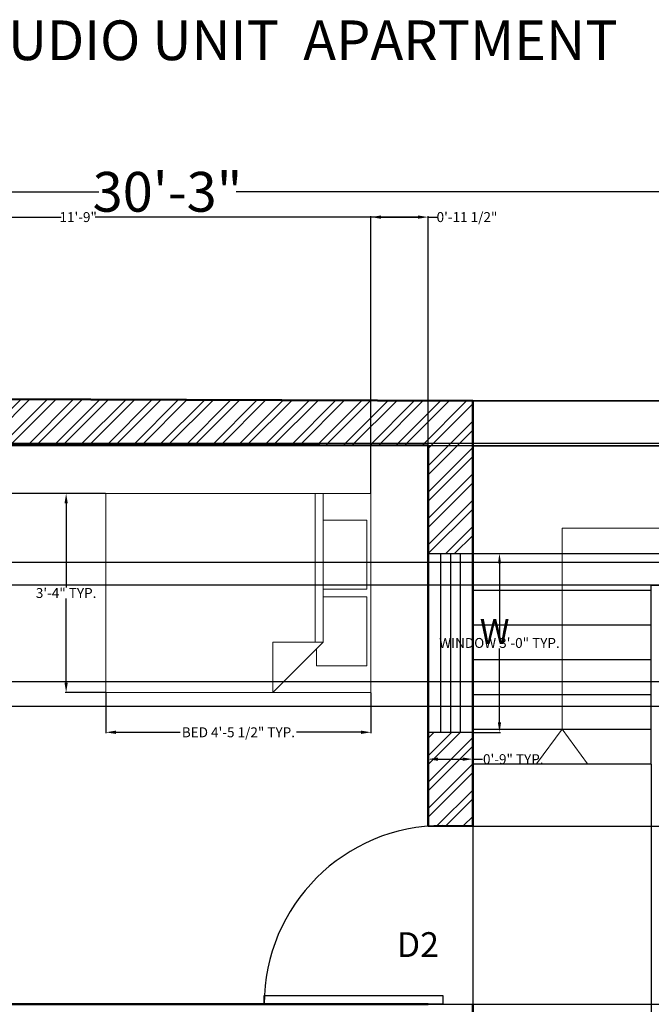
# Model space of a CAD drawing. Units: inches. Extents: x -83 to 408, y 158 to 919.
# Tile 4 of 5: x 111 to 238, y 721 to 919. Entities that reach past the tile are written whole.
import ezdxf

# ---------------------------------------------------------------- set-up
doc = ezdxf.new("R2010")
doc.units = ezdxf.units.IN
doc.header["$MEASUREMENT"] = 0
for name, color, linetype, lineweight in [('A-ANNO-DIMS', 2, 'Continuous', 18), ('A-ANNO-SYMB', 3, 'Continuous', 18), ('A-ANNO-TEXT', 7, 'Continuous', 18), ('A-ANNO-TITL', 7, 'Continuous', 35), ('A-DOOR', 3, 'Continuous', 25), ('A-FLOR-STRS', 7, 'Continuous', 25), ('A-FURN', 8, 'Continuous', 18), ('A-GLAZ', 4, 'Continuous', 25), ('A-WALL', 7, 'Continuous', 50), ('A-WALL-PATT', 252, 'Continuous', 13), ('L-WALL', 7, 'Continuous', 35)]:
    doc.layers.add(name, color=color, linetype=linetype, lineweight=lineweight)
doc.styles.get("Standard").update_dxf_attribs({"font": 'arial.ttf'})
doc.dimstyles.get("Standard").update_dxf_attribs({"dimtxt": 2, "dimasz": 2, "dimexe": 0.18, "dimexo": 0.0625, "dimgap": 0.09, "dimtad": 0, "dimtih": 1, "dimtoh": 1, "dimdec": 0, "dimzin": 0, "dimdsep": 46, "dimlunit": 3, "dimtxsty": 'Standard', "dimcen": 0.09, "dimadec": 0, "dimazin": 0, "dimtfac": 1, "dimtdec": 0, "dimtofl": 0, "dimtmove": 0, "dimatfit": 3, "dimfxl": 1, "dimtolj": 1, "dimtzin": 0, "dimarcsym": 0})

# ---------------------------------------------------------------- blocks, each defined once
blk = doc.blocks.new('Bed - Queen')
for p, q in [((0, -80.00003), (0, 0)), ((0, 0), (59.99999, 0)), ((59.99999, 0), (59.99999, -80.00003)), ((7.99999, -1.2), (28.79998, -1.2)), ((7.99999, -14.4), (7.99999, -1.2)), ((28.79998, -1.2), (28.79998, -14.4)), ((31.19999, -1.2), (51.99999, -1.2)), ((31.19999, -14.4), (31.19999, -1.2)), ((51.99999, -1.2), (51.99999, -16.4)), ((0, -14.4), (44.8, -14.4)), ((59.99999, -29.6), (44.8, -14.4)), ((44.8, -14.4), (44.8, -29.6)), ((44.8, -16.8), (0, -16.8)), ((51.99999, -16.4), (46.79936, -16.4)), ((44.8, -29.6), (59.99999, -29.6)), ((59.99999, -80.00003), (0, -80.00003))]:
    blk.add_line(p, q)
blk = doc.blocks.new('*U13')
for p, q in [((0, 0), (0, -6)), ((36, 0), (36, -6))]:
    blk.add_line(p, q)
blk.add_lwpolyline([(0, 0), (0, 36), (1.75, 36), (1.75, 0)], close=True)
blk.add_arc((0, 0), 36, 0, 90)
blk = doc.blocks.new('*D18')
at = {"layer": 'A-ANNO-DIMS', "color": 0, "lineweight": -2, "transparency": 16777216}
for p, q in [((-40.81, 843.26), (-40.81, 884.97)), ((-38.81, 884.79), (126.86, 884.79)), ((320.19, 884.79), (154.52, 884.79)), ((322.19, 842.73), (322.19, 884.97))]:
    blk.add_line(p, q, dxfattribs=at)
at = {"layer": 'A-ANNO-DIMS', "color": 0, "transparency": 16777216}
for points in [[(-38.81, 885.12), (-38.81, 884.46), (-40.81, 884.79)], [(320.19, 885.12), (320.19, 884.46), (322.19, 884.79)]]:
    blk.add_solid(points, dxfattribs=at)
at = {"layer": 'Defpoints', "color": 0, "transparency": 16777216}
for p in [(322.19, 884.79), (-40.81, 843.2), (322.19, 842.67)]:
    blk.add_point(p, dxfattribs=at)
at = {"layer": 'A-ANNO-DIMS', "color": 0, "transparency": 16777216, "insert": (140.69, 884.79), "char_height": 2, "attachment_point": 5}
blk.add_mtext('\\A1;{\\H4x;30\'-3"}', dxfattribs=at)
blk = doc.blocks.new('WINDOW-36IN')
for p, q in [((2.5, 36), (2.5, 0)), ((4.5, 36), (4.5, 0)), ((6.5, 36), (6.5, 0))]:
    blk.add_line(p, q)
blk.add_lwpolyline([(0, 36), (9, 36), (9, 0), (0, 0)], close=True)
blk = doc.blocks.new('*D23')
at = {"layer": 'A-ANNO-DIMS', "color": 0, "lineweight": -2, "transparency": 16777216}
for p, q in [((202.25, 811.95), (207.77, 811.95)), ((207.59, 809.95), (207.59, 795.08)), ((207.59, 777.95), (207.59, 792.82)), ((202.25, 775.95), (207.77, 775.95))]:
    blk.add_line(p, q, dxfattribs=at)
at = {"layer": 'A-ANNO-DIMS', "color": 0, "transparency": 16777216}
for points in [[(207.26, 809.95), (207.92, 809.95), (207.59, 811.95)], [(207.26, 777.95), (207.92, 777.95), (207.59, 775.95)]]:
    blk.add_solid(points, dxfattribs=at)
at = {"layer": 'Defpoints', "color": 0, "transparency": 16777216}
for p in [(202.19, 811.95), (207.59, 811.95), (202.19, 775.95)]:
    blk.add_point(p, dxfattribs=at)
at = {"layer": 'A-ANNO-DIMS', "color": 0, "transparency": 16777216, "insert": (207.59, 793.95), "char_height": 2, "attachment_point": 5}
blk.add_mtext('\\A1;WINDOW 3\'-0" TYP.', dxfattribs=at)
blk = doc.blocks.new('*D24')
at = {"layer": 'A-ANNO-DIMS', "color": 0, "lineweight": -2, "transparency": 16777216}
for p, q in [((193.19, 775.89), (193.19, 770.37)), ((202.19, 775.89), (202.19, 770.37)), ((195.19, 770.55), (200.19, 770.55)), ((202.19, 770.55), (204.19, 770.55))]:
    blk.add_line(p, q, dxfattribs=at)
at = {"layer": 'A-ANNO-DIMS', "color": 0, "transparency": 16777216}
for points in [[(195.19, 770.88), (195.19, 770.22), (193.19, 770.55)], [(200.19, 770.88), (200.19, 770.22), (202.19, 770.55)]]:
    blk.add_solid(points, dxfattribs=at)
at = {"layer": 'Defpoints', "color": 0, "transparency": 16777216}
for p in [(193.19, 775.95), (202.19, 775.95), (202.19, 770.55)]:
    blk.add_point(p, dxfattribs=at)
at = {"layer": 'A-ANNO-DIMS', "color": 0, "transparency": 16777216, "insert": (210.37, 770.55), "char_height": 2, "attachment_point": 5}
blk.add_mtext('\\A1;0\'-9" TYP.', dxfattribs=at)
blk = doc.blocks.new('*D31')
at = {"layer": 'A-ANNO-DIMS', "color": 0, "lineweight": -2, "transparency": 16777216}
for p, q in [((128.28, 783.91), (128.28, 775.78)), ((181.69, 783.91), (181.69, 775.78)), ((130.28, 775.96), (143.25, 775.96)), ((179.69, 775.96), (166.71, 775.96))]:
    blk.add_line(p, q, dxfattribs=at)
at = {"layer": 'A-ANNO-DIMS', "color": 0, "transparency": 16777216}
for points in [[(130.28, 776.3), (130.28, 775.63), (128.28, 775.96)], [(179.69, 776.3), (179.69, 775.63), (181.69, 775.96)]]:
    blk.add_solid(points, dxfattribs=at)
at = {"layer": 'Defpoints', "color": 0, "transparency": 16777216}
for p in [(128.28, 783.98), (181.69, 783.98), (181.69, 775.96)]:
    blk.add_point(p, dxfattribs=at)
at = {"layer": 'A-ANNO-DIMS', "color": 0, "transparency": 16777216, "insert": (154.98, 775.96), "char_height": 2, "attachment_point": 5}
blk.add_mtext('\\A1;BED 4\'-5 1/2" TYP.', dxfattribs=at)
blk = doc.blocks.new('*D32')
at = {"layer": 'A-ANNO-DIMS', "color": 0, "lineweight": -2, "transparency": 16777216}
for p, q in [((128.21, 824.04), (120.08, 824.04)), ((120.26, 822.04), (120.26, 805.12)), ((120.26, 785.98), (120.26, 802.89)), ((128.21, 783.98), (120.08, 783.98))]:
    blk.add_line(p, q, dxfattribs=at)
at = {"layer": 'A-ANNO-DIMS', "color": 0, "transparency": 16777216}
for points in [[(119.93, 822.04), (120.6, 822.04), (120.26, 824.04)], [(119.93, 785.98), (120.6, 785.98), (120.26, 783.98)]]:
    blk.add_solid(points, dxfattribs=at)
at = {"layer": 'Defpoints', "color": 0, "transparency": 16777216}
for p in [(128.28, 824.04), (120.26, 783.98), (128.28, 783.98)]:
    blk.add_point(p, dxfattribs=at)
at = {"layer": 'A-ANNO-DIMS', "color": 0, "transparency": 16777216, "insert": (120.26, 804.01), "char_height": 2, "attachment_point": 5}
blk.add_mtext('\\A1;3\'-4" TYP.', dxfattribs=at)
blk = doc.blocks.new('*D48')
at = {"layer": 'A-ANNO-DIMS', "color": 0, "lineweight": -2, "transparency": 16777216}
for p, q in [((47.25, 834.2), (358.87, 834.2)), ((358.69, 832.2), (358.69, 811.31)), ((358.69, 788.2), (358.69, 809.09)), ((47.25, 786.2), (358.87, 786.2))]:
    blk.add_line(p, q, dxfattribs=at)
at = {"layer": 'A-ANNO-DIMS', "color": 0, "transparency": 16777216}
for points in [[(358.36, 832.2), (359.02, 832.2), (358.69, 834.2)], [(358.36, 788.2), (359.02, 788.2), (358.69, 786.2)]]:
    blk.add_solid(points, dxfattribs=at)
at = {"layer": 'Defpoints', "color": 0, "transparency": 16777216}
for p in [(47.19, 834.2), (47.19, 786.2), (358.69, 786.2)]:
    blk.add_point(p, dxfattribs=at)
at = {"layer": 'A-ANNO-DIMS', "color": 0, "transparency": 16777216, "insert": (358.69, 810.2), "char_height": 2, "attachment_point": 5}
blk.add_mtext('\\A1;4\'-0"', dxfattribs=at)
blk = doc.blocks.new('*D49')
at = {"layer": 'A-ANNO-DIMS', "color": 0, "lineweight": -2, "transparency": 16777216}
for p, q in [((47.25, 810.2), (358.87, 810.2)), ((358.69, 808.2), (358.69, 799.31)), ((358.69, 788.2), (358.69, 797.09)), ((47.25, 786.2), (358.87, 786.2))]:
    blk.add_line(p, q, dxfattribs=at)
at = {"layer": 'A-ANNO-DIMS', "color": 0, "transparency": 16777216}
for points in [[(358.36, 808.2), (359.02, 808.2), (358.69, 810.2)], [(358.36, 788.2), (359.02, 788.2), (358.69, 786.2)]]:
    blk.add_solid(points, dxfattribs=at)
at = {"layer": 'Defpoints', "color": 0, "transparency": 16777216}
for p in [(47.19, 810.2), (47.19, 786.2), (358.69, 786.2)]:
    blk.add_point(p, dxfattribs=at)
at = {"layer": 'A-ANNO-DIMS', "color": 0, "transparency": 16777216, "insert": (358.69, 798.2), "char_height": 2, "attachment_point": 5}
blk.add_mtext('\\A1;2\'-0"', dxfattribs=at)
blk = doc.blocks.new('*D50')
at = {"layer": 'A-ANNO-DIMS', "color": 0, "lineweight": -2, "transparency": 16777216}
for p, q in [((193.25, 757.08), (358.87, 757.08)), ((358.69, 755.08), (358.69, 740.25)), ((358.69, 723.2), (358.69, 738.03)), ((193.25, 721.2), (358.87, 721.2))]:
    blk.add_line(p, q, dxfattribs=at)
at = {"layer": 'A-ANNO-DIMS', "color": 0, "transparency": 16777216}
for points in [[(358.36, 755.08), (359.02, 755.08), (358.69, 757.08)], [(358.36, 723.2), (359.02, 723.2), (358.69, 721.2)]]:
    blk.add_solid(points, dxfattribs=at)
at = {"layer": 'Defpoints', "color": 0, "transparency": 16777216}
for p in [(193.19, 757.08), (193.19, 721.2), (358.69, 721.2)]:
    blk.add_point(p, dxfattribs=at)
at = {"layer": 'A-ANNO-DIMS', "color": 0, "transparency": 16777216, "insert": (358.69, 739.14), "char_height": 2, "attachment_point": 5}
blk.add_mtext('\\A1;3\'-0"', dxfattribs=at)
blk = doc.blocks.new('*D51')
at = {"layer": 'A-ANNO-DIMS', "color": 0, "lineweight": -2, "transparency": 16777216}
for p, q in [((52.19, 834.26), (52.19, 879.88)), ((54.19, 879.7), (119.26, 879.7)), ((191.19, 879.7), (126.12, 879.7)), ((193.19, 833.76), (193.19, 879.88))]:
    blk.add_line(p, q, dxfattribs=at)
at = {"layer": 'A-ANNO-DIMS', "color": 0, "transparency": 16777216}
for points in [[(54.19, 880.03), (54.19, 879.37), (52.19, 879.7)], [(191.19, 880.03), (191.19, 879.37), (193.19, 879.7)]]:
    blk.add_solid(points, dxfattribs=at)
at = {"layer": 'Defpoints', "color": 0, "transparency": 16777216}
for p in [(193.19, 879.7), (52.19, 834.2), (193.19, 833.7)]:
    blk.add_point(p, dxfattribs=at)
at = {"layer": 'A-ANNO-DIMS', "color": 0, "transparency": 16777216, "insert": (122.69, 879.7), "char_height": 2, "attachment_point": 5}
blk.add_mtext('\\A1;11\'-9"', dxfattribs=at)
blk = doc.blocks.new('*D54')
at = {"layer": 'A-ANNO-DIMS', "color": 0, "lineweight": -2, "transparency": 16777216}
for p, q in [((193.25, 833.7), (358.87, 833.7)), ((358.69, 831.7), (358.69, 823.94)), ((358.69, 813.95), (358.69, 821.71)), ((193.25, 811.95), (358.87, 811.95))]:
    blk.add_line(p, q, dxfattribs=at)
at = {"layer": 'A-ANNO-DIMS', "color": 0, "transparency": 16777216}
for points in [[(358.36, 831.7), (359.02, 831.7), (358.69, 833.7)], [(358.36, 813.95), (359.02, 813.95), (358.69, 811.95)]]:
    blk.add_solid(points, dxfattribs=at)
at = {"layer": 'Defpoints', "color": 0, "transparency": 16777216}
for p in [(193.19, 833.7), (193.19, 811.95), (358.69, 811.95)]:
    blk.add_point(p, dxfattribs=at)
at = {"layer": 'A-ANNO-DIMS', "color": 0, "transparency": 16777216, "insert": (358.69, 822.83), "char_height": 2, "attachment_point": 5}
blk.add_mtext('\\A1;1\'-10"', dxfattribs=at)
blk = doc.blocks.new('*D56')
at = {"layer": 'A-ANNO-DIMS', "color": 0, "lineweight": -2, "transparency": 16777216}
for p, q in [((52.25, 781.2), (358.87, 781.2)), ((358.69, 779.2), (358.69, 752.31)), ((358.69, 723.2), (358.69, 750.09)), ((47.25, 721.2), (358.87, 721.2))]:
    blk.add_line(p, q, dxfattribs=at)
at = {"layer": 'A-ANNO-DIMS', "color": 0, "transparency": 16777216}
for points in [[(358.36, 779.2), (359.02, 779.2), (358.69, 781.2)], [(358.36, 723.2), (359.02, 723.2), (358.69, 721.2)]]:
    blk.add_solid(points, dxfattribs=at)
at = {"layer": 'Defpoints', "color": 0, "transparency": 16777216}
for p in [(52.19, 781.2), (47.19, 721.2), (358.69, 721.2)]:
    blk.add_point(p, dxfattribs=at)
at = {"layer": 'A-ANNO-DIMS', "color": 0, "transparency": 16777216, "insert": (358.69, 751.2), "char_height": 2, "attachment_point": 5}
blk.add_mtext('\\A1;5\'-0"', dxfattribs=at)
blk = doc.blocks.new('*D59')
at = {"layer": 'A-ANNO-DIMS', "color": 0, "lineweight": -2, "transparency": 16777216}
for p, q in [((202.19, 769.53), (202.19, 160.47)), ((238.19, 769.53), (238.19, 160.47)), ((204.19, 160.65), (217.44, 160.65)), ((236.19, 160.65), (222.94, 160.65))]:
    blk.add_line(p, q, dxfattribs=at)
at = {"layer": 'A-ANNO-DIMS', "color": 0, "transparency": 16777216}
for points in [[(204.19, 160.98), (204.19, 160.32), (202.19, 160.65)], [(236.19, 160.98), (236.19, 160.32), (238.19, 160.65)]]:
    blk.add_solid(points, dxfattribs=at)
at = {"layer": 'Defpoints', "color": 0, "transparency": 16777216}
for p in [(202.19, 769.59), (238.19, 769.59), (238.19, 160.65)]:
    blk.add_point(p, dxfattribs=at)
at = {"layer": 'A-ANNO-DIMS', "color": 0, "transparency": 16777216, "insert": (220.19, 160.65), "char_height": 2, "attachment_point": 5}
blk.add_mtext('\\A1;3\'-0"', dxfattribs=at)
blk = doc.blocks.new('*D62')
at = {"layer": 'A-ANNO-DIMS', "color": 0, "lineweight": -2, "transparency": 16777216}
for p, q in [((272.31, 833.67), (-77.49, 833.67)), ((-77.31, 831.67), (-77.31, 820.72)), ((-77.31, 807.59), (-77.31, 818.54)), ((274.13, 805.59), (-77.49, 805.59))]:
    blk.add_line(p, q, dxfattribs=at)
at = {"layer": 'A-ANNO-DIMS', "color": 0, "transparency": 16777216}
for points in [[(-77.64, 831.67), (-76.98, 831.67), (-77.31, 833.67)], [(-77.64, 807.59), (-76.98, 807.59), (-77.31, 805.59)]]:
    blk.add_solid(points, dxfattribs=at)
at = {"layer": 'Defpoints', "color": 0, "transparency": 16777216}
for p in [(-77.31, 833.67), (272.37, 833.67), (274.19, 805.59)]:
    blk.add_point(p, dxfattribs=at)
at = {"layer": 'A-ANNO-DIMS', "color": 0, "transparency": 16777216, "insert": (-77.31, 819.63), "char_height": 2, "attachment_point": 5}
blk.add_mtext('\\A1;2\'-4"', dxfattribs=at)
blk = doc.blocks.new('*D71')
at = {"layer": 'A-ANNO-DIMS', "color": 0, "lineweight": -2, "transparency": 16777216}
for p, q in [((181.69, 824.1), (181.69, 879.88)), ((183.69, 879.7), (191.19, 879.7)), ((193.19, 833.76), (193.19, 879.88)), ((193.19, 879.7), (195.19, 879.7))]:
    blk.add_line(p, q, dxfattribs=at)
at = {"layer": 'A-ANNO-DIMS', "color": 0, "transparency": 16777216}
for points in [[(183.69, 880.03), (183.69, 879.37), (181.69, 879.7)], [(191.19, 880.03), (191.19, 879.37), (193.19, 879.7)]]:
    blk.add_solid(points, dxfattribs=at)
at = {"layer": 'Defpoints', "color": 0, "transparency": 16777216}
for p in [(193.19, 879.7), (193.19, 833.7), (181.69, 824.04)]:
    blk.add_point(p, dxfattribs=at)
at = {"layer": 'A-ANNO-DIMS', "color": 0, "transparency": 16777216, "insert": (201.04, 879.7), "char_height": 2, "attachment_point": 5}
blk.add_mtext('\\A1;0\'-11 1/2"', dxfattribs=at)
blk = doc.blocks.new('*D72')
at = {"layer": 'A-ANNO-DIMS', "color": 0, "lineweight": -2, "transparency": 16777216}
for p, q in [((193.13, 833.7), (-77.49, 833.7)), ((-77.31, 831.7), (-77.31, 829.99)), ((-77.31, 826.04), (-77.31, 827.74)), ((128.21, 824.04), (-77.49, 824.04))]:
    blk.add_line(p, q, dxfattribs=at)
at = {"layer": 'A-ANNO-DIMS', "color": 0, "transparency": 16777216}
for points in [[(-77.64, 831.7), (-76.98, 831.7), (-77.31, 833.7)], [(-77.64, 826.04), (-76.98, 826.04), (-77.31, 824.04)]]:
    blk.add_solid(points, dxfattribs=at)
at = {"layer": 'Defpoints', "color": 0, "transparency": 16777216}
for p in [(-77.31, 833.7), (193.19, 833.7), (128.28, 824.04)]:
    blk.add_point(p, dxfattribs=at)
at = {"layer": 'A-ANNO-DIMS', "color": 0, "transparency": 16777216, "insert": (-77.31, 828.87), "char_height": 2, "attachment_point": 5}
blk.add_mtext('\\A1;0\'-9 1/2"', dxfattribs=at)

msp = doc.modelspace()

# ---------------------------------------------------------------- hatches: boundary and pattern name
at = {"layer": 'A-WALL-PATT'}
h = msp.add_hatch(dxfattribs=at)
h.set_pattern_fill('ANSI32', color=256, scale=10)
h.paths.add_polyline_path([(202.19, 842.67), (52.21, 843.2), (-40.81, 843.2), (-40.81, 814.39), (-31.81, 814.39), (-31.81, 834.2), (47.19, 834.2), (47.19, 810.2), (52.19, 810.2), (52.19, 834.2), (193.19, 833.7), (193.19, 811.95), (202.19, 811.95)])
h.paths.add_polyline_path([(-31.81, 781.2), (52.19, 781.2), (52.19, 786.2), (46.19, 786.2), (22.19, 786.2), (-31.81, 786.2), (-31.81, 802.39), (-40.81, 802.39), (-40.81, 771.16), (-31.81, 771.16)])
h.paths.add_polyline_path([(-31.81, 735.16), (-40.81, 735.16), (-40.81, 721.18), (-31.81, 721.18)])
h.paths.add_polyline_path([(202.19, 775.95), (193.19, 775.95), (193.19, 757.08, -0.020861), (196.19, 757.2), (202.19, 757.2)])

# ---------------------------------------------------------------- linework, layer by layer
at = {"layer": 'A-ANNO-SYMB'}
for p, q in [((220.19, 776.59), (220.19, 817.05)), ((220.19, 817.05), (291.39, 817.05))]:
    msp.add_line(p, q, dxfattribs=at)
msp.add_lwpolyline([(220.19, 776.59), (215.07, 769.59), (225.31, 769.59)], close=True, dxfattribs=at)
at = {"layer": 'A-FLOR-STRS'}
for p, q in [((238.19, 769.59), (238.19, 805.59)), ((238.19, 805.59), (274.19, 805.59)), ((202.19, 804.59), (238.19, 804.59)), ((202.19, 797.59), (238.19, 797.59)), ((202.19, 790.59), (238.19, 790.59)), ((202.19, 783.59), (238.19, 783.59)), ((202.19, 776.59), (238.19, 776.59)), ((202.19, 769.59), (238.19, 769.59))]:
    msp.add_line(p, q, dxfattribs=at)
at = {"layer": 'A-WALL'}
for p, q in [((202.19, 842.67), (52.22, 843.2)), ((202.19, 757.2), (202.19, 842.67)), ((193.19, 833.7), (52.19, 834.2)), ((193.19, 757.08), (193.19, 833.7)), ((47.19, 721.2), (193.19, 721.2)), ((202.19, 712.2), (202.19, 721.2))]:
    msp.add_line(p, q, dxfattribs=at)
at = {"layer": 'L-WALL'}
for p, q in [((322.19, 842.67), (202.19, 842.67)), ((202.19, 842.67), (202.19, 842.67)), ((202.19, 833.67), (313.19, 833.67))]:
    msp.add_line(p, q, dxfattribs=at)

# ---------------------------------------------------------------- block references
at = {"layer": 'A-DOOR', "rotation": 90}
msp.add_blockref('*U13', (196.19, 721.2), dxfattribs=at)
at = {"layer": 'A-FURN', "xscale": 0.667678018977486, "yscale": 0.667678018977486, "zscale": 0.667678018977486, "rotation": 270}
msp.add_blockref('Bed - Queen', (181.69, 824.04), dxfattribs=at)
at = {"layer": 'A-GLAZ'}
msp.add_blockref('WINDOW-36IN', (193.19, 775.95), dxfattribs=at)

# ---------------------------------------------------------------- texts
at = {"layer": 'A-ANNO-TEXT', "char_height": 5, "attachment_point": 1}
for s, width, insert in [('W', 4.9358, (203.62, 798.76)), ('D2', 13.3697, (186.91, 735.71))]:
    msp.add_mtext_dynamic_manual_height_columns(s, width=width, gutter_width=1, heights=[0], dxfattribs=dict(at, insert=insert))
at = {"layer": 'A-ANNO-TITL', "insert": (95.49, 919.3), "char_height": 8, "attachment_point": 1}
msp.add_mtext_dynamic_manual_height_columns('STUDIO UNIT  APARTMENT', width=288.4341, gutter_width=1, heights=[0], dxfattribs=at)

# ---------------------------------------------------------------- dimensions: what is measured, and where the dimension line sits
at = {"layer": 'A-ANNO-DIMS'}
for base, p1, p2, text, override, picture, middle in [((322.19, 884.79), (-40.81, 843.2), (322.19, 842.67), '{\\H4x;<>}', {"dimclrd": 0, "dimclre": 0, "dimclrt": 0}, '*D18', (140.69, 884.79)), ((181.69, 775.96), (128.28, 783.98), (181.69, 783.98), 'BED <> TYP.', {"dimdec": 1, "dimlfac": 1, "dimrnd": 0, "dimzin": 1, "dimdsep": 46, "dimlunit": 4, "dimfrac": 2}, '*D31', (154.98, 775.96)), ((202.19, 770.55), (193.19, 775.95), (202.19, 775.95), '<> TYP.', {"dimdec": 1, "dimlfac": 1, "dimrnd": 0, "dimzin": 1, "dimdsep": 46, "dimlunit": 4, "dimfrac": 2}, '*D24', (210.37, 770.55))]:
    dim = msp.add_linear_dim(base=base, p1=p1, p2=p2, text=text, dimstyle='Standard', override=override, dxfattribs=at)
    dim.commit()
    dim.dimension.update_dxf_attribs({"geometry": picture, "text_midpoint": middle})
for base, p1, p2, picture, middle in [((193.19, 879.7), (181.69, 824.04), (193.19, 833.7), '*D71', (201.04, 879.7)), ((193.19, 879.7), (52.19, 834.2), (193.19, 833.7), '*D51', (122.69, 879.7)), ((238.19, 160.65), (202.19, 769.59), (238.19, 769.59), '*D59', (220.19, 160.65))]:
    dim = msp.add_linear_dim(base=base, p1=p1, p2=p2, dimstyle='Standard', override={"dimdec": 1, "dimlfac": 1, "dimrnd": 0, "dimzin": 1, "dimdsep": 46, "dimlunit": 4, "dimfrac": 2}, dxfattribs=at)
    dim.commit()
    dim.dimension.update_dxf_attribs({"geometry": picture, "text_midpoint": middle})
for base, p1, p2, picture, middle in [((-77.31, 833.7), (128.28, 824.04), (193.19, 833.7), '*D72', (-77.31, 828.87)), ((-77.31, 833.67), (274.19, 805.59), (272.37, 833.67), '*D62', (-77.31, 819.63)), ((358.69, 786.2), (47.19, 834.2), (47.19, 786.2), '*D48', (358.69, 810.2)), ((358.6891, 811.95026), (193.1891, 833.70029), (193.1891, 811.95026), '*D54', (358.6891, 822.82528)), ((358.69, 786.2), (47.19, 810.2), (47.19, 786.2), '*D49', (358.69, 798.2)), ((358.69, 721.2), (52.19, 781.2), (47.19, 721.2), '*D56', (358.69, 751.2)), ((358.69, 721.2), (193.19, 757.08), (193.19, 721.2), '*D50', (358.69, 739.14))]:
    dim = msp.add_linear_dim(base=base, p1=p1, p2=p2, angle=90, dimstyle='Standard', override={"dimdec": 1, "dimlfac": 1, "dimrnd": 0, "dimzin": 1, "dimdsep": 46, "dimlunit": 4, "dimfrac": 2}, dxfattribs=at)
    dim.commit()
    dim.dimension.update_dxf_attribs({"geometry": picture, "text_midpoint": middle})
for base, p1, p2, angle, text, picture, middle in [((120.26, 783.98), (128.28, 824.04), (128.28, 783.98), 270, '<> TYP.', '*D32', (120.26, 804.01)), ((207.59, 811.95), (202.19, 775.95), (202.19, 811.95), 90, 'WINDOW <> TYP.', '*D23', (207.59, 793.95))]:
    dim = msp.add_linear_dim(base=base, p1=p1, p2=p2, angle=angle, text=text, dimstyle='Standard', override={"dimdec": 1, "dimlfac": 1, "dimrnd": 0, "dimzin": 1, "dimdsep": 46, "dimlunit": 4, "dimfrac": 2}, dxfattribs=at)
    dim.commit()
    dim.dimension.update_dxf_attribs({"geometry": picture, "text_midpoint": middle})

doc.saveas('drawing.dxf')
